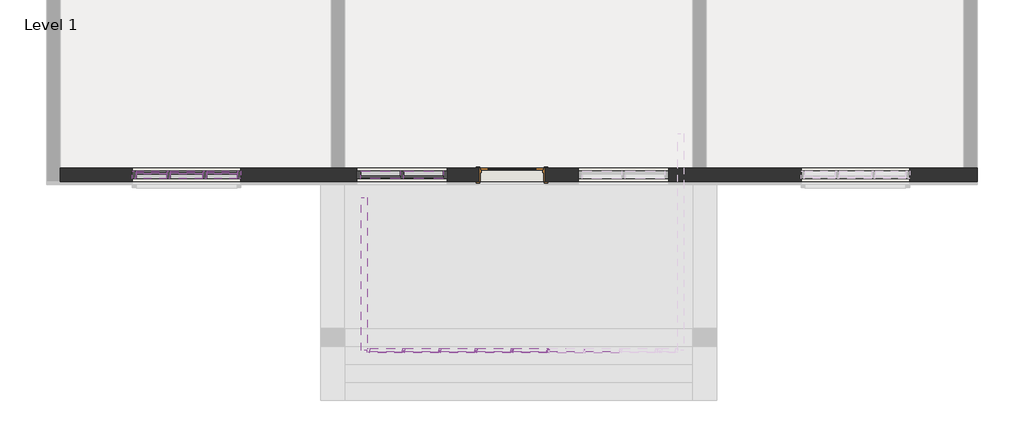
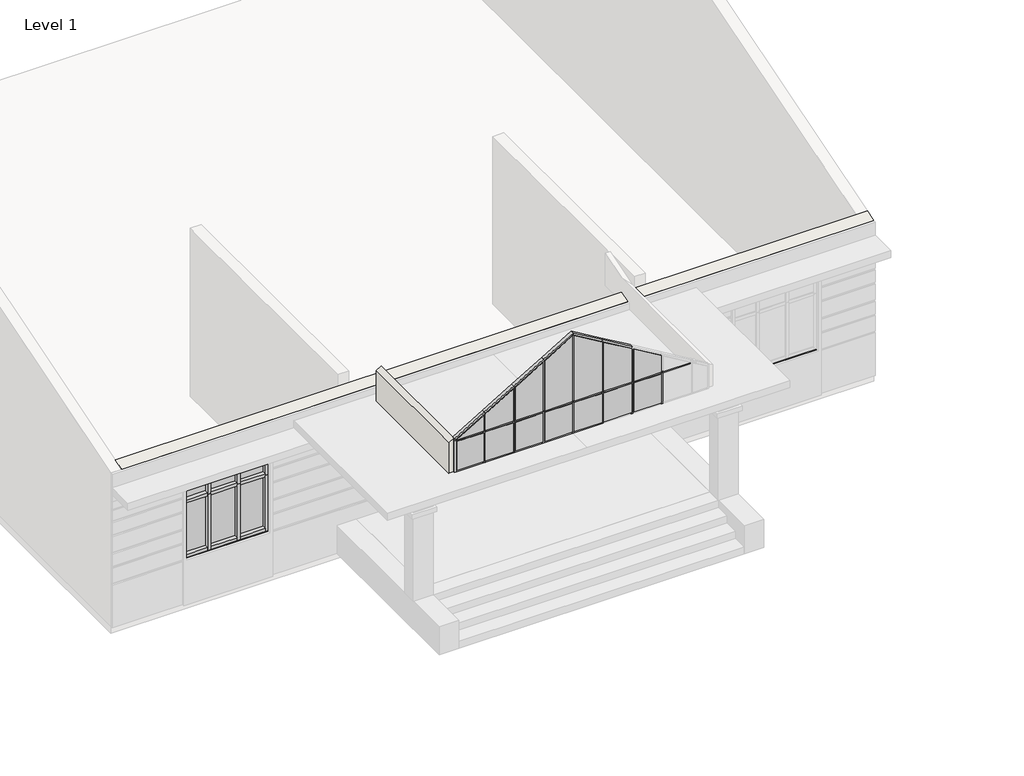
# One storey, part 1 of 2: 57 members, 22 plates, 2 walls, 1 door.
"""IFC4 building model written with IfcOpenShell, lengths in millimetres."""

from ifc_helpers import new_model, si_unit, frame, origin, place, context, project, spatial, polyline, outline, extrude, faceted_brep, transform, mapped, element, save
from components import door_103cf79b, member_83e1ecc3, member_06c20982, member_b8e7570c, member_bb410062, member_6458fcce, member_a67f877f, member_c8158400, member_1ba99afd, member_594eddbe, member_3c184fc8, member_ff75f20c, member_eb314aa0, member_ee25ef0f, member_c8c782b1, member_99569e28, member_7b64f847, member_0b7646a3, member_2b49869a, member_aaa03826, member_0a1a1ade, member_a980948f, member_6e77e263, member_47bfaf8a, member_75074519, member_c33c434a, member_38e9bff8, member_062c1ce8, system_panel_glazed_d796fc41, system_panel_glazed_2d0a2ff2, system_panel_glazed_c086748d, system_panel_glazed_4278ab3a, system_panel_glazed_31f7001e, system_panel_glazed_f02c31ce, system_panel_glazed_0f57d06b, system_panel_glazed_ee2a426c, system_panel_glazed_65593f79, system_panel_glazed_0e80e67f, system_panel_glazed_cec062fa, system_panel_glazed_9c640d8a, system_panel_glazed_3d703fd1, system_panel_glazed_02eac8f9

model = new_model("IFC4")

# Units and contexts
model_context = context("Model", 3, world=origin())
ifc_project = project(units=[si_unit("LENGTHUNIT", "METRE", prefix="MILLI")], contexts=[model_context])

# Site, building, storey
site = spatial("IfcSite", under=ifc_project)
building = spatial("IfcBuilding", under=site)
storey = spatial("IfcBuildingStorey", under=building, Name="Level 1", Elevation=0.0)

# Door
placement = place(None, origin())
door_shape = door_103cf79b(model_context)
element("IfcDoor", 1, ObjectType="Door-Interior-Single-1_Panel-Wood : 3'6\" x 7'", at=placement, inside=storey, context=model_context, shape_type="MappedRepresentation", body=[
    mapped(door_shape, transform((-905.7652342, -1559.6844336, 584.2), x_axis=(1.0, 0.0, 0.0), y_axis=(0.0, 1.0, 0.0), z_axis=(0.0, 0.0, 1.0))),
])

# Members
member_shape = member_83e1ecc3(model_context)
element("IfcMember", 2, ObjectType="Rectangular Mullion : 1.5\" x 2.5\" rectangular", at=placement, inside=storey, context=model_context, shape_type="MappedRepresentation", body=[
    mapped(member_shape, transform((-905.7652342, -4522.7940778, 5385.8290246), x_axis=(0.5109163571310298, 0.0, 0.8596304299034313), y_axis=(0.0, 1.0, 0.0), z_axis=(-0.8596304299034313, 0.0, 0.5109163571310298))),
])
member_2_shape = member_06c20982(model_context)
element("IfcMember", 3, ObjectType="Rectangular Mullion : 1.5\" x 2.5\" rectangular", at=placement, inside=storey, context=model_context, shape_type="MappedRepresentation", body=[
    mapped(member_2_shape, transform((-3345.0817556, -4522.7940778, 3936.0354067), x_axis=(-0.5109163571310278, 0.0, 0.8596304299034325), y_axis=(0.0, 1.0, 0.0), z_axis=(-0.8596304299034324, 0.0, -0.5109163571310277))),
])
member_3_shape = member_b8e7570c(model_context)
element("IfcMember", 4, ObjectType="Rectangular Mullion : 1.5\" x 2.5\" rectangular", at=placement, inside=storey, context=model_context, shape_type="MappedRepresentation", body=[
    mapped(member_3_shape, transform((-1496.3152342, -4522.7940778, 3886.2), x_axis=(0.0, 0.0, 1.0), y_axis=(0.0, 1.0, 0.0), z_axis=(-1.0, 0.0, 0.0))),
])
element("IfcMember", 5, ObjectType="Rectangular Mullion : 1.5\" x 2.5\" rectangular", at=placement, inside=storey, context=model_context, shape_type="MappedRepresentation", body=[
    mapped(member_3_shape, transform((-886.7152342, -4522.7940778, 3886.2), x_axis=(0.0, 0.0, 1.0), y_axis=(0.0, 1.0, 0.0), z_axis=(-1.0, 0.0, 0.0))),
])
element("IfcMember", 6, ObjectType="Rectangular Mullion : 1.5\" x 2.5\" rectangular", at=placement, inside=storey, context=model_context, shape_type="MappedRepresentation", body=[
    mapped(member_3_shape, transform((-277.1152342, -4522.7940778, 3886.2), x_axis=(0.0, 0.0, 1.0), y_axis=(0.0, 1.0, 0.0), z_axis=(-1.0, 0.0, 0.0))),
])
element("IfcMember", 7, ObjectType="Rectangular Mullion : 1.5\" x 2.5\" rectangular", at=placement, inside=storey, context=model_context, shape_type="MappedRepresentation", body=[
    mapped(member_3_shape, transform((332.4847658, -4522.7940778, 3886.2), x_axis=(0.0, 0.0, 1.0), y_axis=(0.0, 1.0, 0.0), z_axis=(-1.0, 0.0, 0.0))),
])
element("IfcMember", 8, ObjectType="Rectangular Mullion : 1.5\" x 2.5\" rectangular", at=placement, inside=storey, context=model_context, shape_type="MappedRepresentation", body=[
    mapped(member_3_shape, transform((942.0847658, -4522.7940778, 3886.2), x_axis=(0.0, 0.0, 1.0), y_axis=(0.0, 1.0, 0.0), z_axis=(-1.0, 0.0, 0.0))),
])
element("IfcMember", 9, ObjectType="Rectangular Mullion : 1.5\" x 2.5\" rectangular", at=placement, inside=storey, context=model_context, shape_type="MappedRepresentation", body=[
    mapped(member_3_shape, transform((-2105.9152342, -4522.7940778, 3886.2), x_axis=(0.0, 0.0, 1.0), y_axis=(0.0, 1.0, 0.0), z_axis=(-1.0, 0.0, 0.0))),
])
element("IfcMember", 10, ObjectType="Rectangular Mullion : 1.5\" x 2.5\" rectangular", at=placement, inside=storey, context=model_context, shape_type="MappedRepresentation", body=[
    mapped(member_3_shape, transform((-2715.5152342, -4522.7940778, 3886.2), x_axis=(0.0, 0.0, 1.0), y_axis=(0.0, 1.0, 0.0), z_axis=(-1.0, 0.0, 0.0))),
])
member_4_shape = member_bb410062(model_context)
element("IfcMember", 11, ObjectType="Rectangular Mullion : 1.5\" x 2.5\" rectangular", at=placement, inside=storey, context=model_context, shape_type="MappedRepresentation", body=[
    mapped(member_4_shape, transform((-3306.9817556, -4522.7940778, 3886.2), x_axis=(0.0, 0.0, 1.0), y_axis=(0.0, 1.0, 0.0), z_axis=(-1.0, 0.0, 0.0))),
])
member_5_shape = member_6458fcce(model_context)
element("IfcMember", 12, ObjectType="Rectangular Mullion : 1.5\" x 2.5\" rectangular", at=placement, inside=storey, context=model_context, shape_type="MappedRepresentation", body=[
    mapped(member_5_shape, transform((-905.7652342, -4522.7940778, 3200.4), x_axis=(-1.0, 0.0, 0.0), y_axis=(0.0, 1.0, 0.0), z_axis=(0.0, 0.0, -1.0))),
])
element("IfcMember", 13, ObjectType="Rectangular Mullion : 1.5\" x 2.5\" rectangular", at=placement, inside=storey, context=model_context, shape_type="MappedRepresentation", body=[
    mapped(member_5_shape, transform((-296.1652342, -4522.7940778, 3200.4), x_axis=(-1.0, 0.0, 0.0), y_axis=(0.0, 1.0, 0.0), z_axis=(0.0, 0.0, -1.0))),
])
element("IfcMember", 14, ObjectType="Rectangular Mullion : 1.5\" x 2.5\" rectangular", at=placement, inside=storey, context=model_context, shape_type="MappedRepresentation", body=[
    mapped(member_5_shape, transform((313.4347658, -4522.7940778, 3200.4), x_axis=(-1.0, 0.0, 0.0), y_axis=(0.0, 1.0, 0.0), z_axis=(0.0, 0.0, -1.0))),
])
element("IfcMember", 15, ObjectType="Rectangular Mullion : 1.5\" x 2.5\" rectangular", at=placement, inside=storey, context=model_context, shape_type="MappedRepresentation", body=[
    mapped(member_5_shape, transform((923.0347658, -4522.7940778, 3200.4), x_axis=(-1.0, 0.0, 0.0), y_axis=(0.0, 1.0, 0.0), z_axis=(0.0, 0.0, -1.0))),
])
element("IfcMember", 16, ObjectType="Rectangular Mullion : 1.5\" x 2.5\" rectangular", at=placement, inside=storey, context=model_context, shape_type="MappedRepresentation", body=[
    mapped(member_5_shape, transform((-1515.3652342, -4522.7940778, 3200.4), x_axis=(-1.0, 0.0, 0.0), y_axis=(0.0, 1.0, 0.0), z_axis=(0.0, 0.0, -1.0))),
])
element("IfcMember", 17, ObjectType="Rectangular Mullion : 1.5\" x 2.5\" rectangular", at=placement, inside=storey, context=model_context, shape_type="MappedRepresentation", body=[
    mapped(member_5_shape, transform((-2124.9652342, -4522.7940778, 3200.4), x_axis=(-1.0, 0.0, 0.0), y_axis=(0.0, 1.0, 0.0), z_axis=(0.0, 0.0, -1.0))),
])
element("IfcMember", 18, ObjectType="Rectangular Mullion : 1.5\" x 2.5\" rectangular", at=placement, inside=storey, context=model_context, shape_type="MappedRepresentation", body=[
    mapped(member_5_shape, transform((-2734.5652342, -4522.7940778, 3200.4), x_axis=(-1.0, 0.0, 0.0), y_axis=(0.0, 1.0, 0.0), z_axis=(0.0, 0.0, -1.0))),
])
member_6_shape = member_a67f877f(model_context)
element("IfcMember", 19, ObjectType="Rectangular Mullion : 1.5\" x 2.5\" rectangular", at=placement, inside=storey, context=model_context, shape_type="MappedRepresentation", body=[
    mapped(member_6_shape, transform((-924.8152342, -4522.7940778, 3200.4), x_axis=(0.0, 0.0, -1.0), y_axis=(0.0, 1.0, 0.0), z_axis=(1.0, 0.0, 0.0))),
])
element("IfcMember", 20, ObjectType="Rectangular Mullion : 1.5\" x 2.5\" rectangular", at=placement, inside=storey, context=model_context, shape_type="MappedRepresentation", body=[
    mapped(member_6_shape, transform((-315.2152342, -4522.7940778, 3200.4), x_axis=(0.0, 0.0, -1.0), y_axis=(0.0, 1.0, 0.0), z_axis=(1.0, 0.0, 0.0))),
])
element("IfcMember", 21, ObjectType="Rectangular Mullion : 1.5\" x 2.5\" rectangular", at=placement, inside=storey, context=model_context, shape_type="MappedRepresentation", body=[
    mapped(member_6_shape, transform((-1534.4152342, -4522.7940778, 3200.4), x_axis=(0.0, 0.0, -1.0), y_axis=(0.0, 1.0, 0.0), z_axis=(1.0, 0.0, 0.0))),
])
element("IfcMember", 22, ObjectType="Rectangular Mullion : 1.5\" x 2.5\" rectangular", at=placement, inside=storey, context=model_context, shape_type="MappedRepresentation", body=[
    mapped(member_6_shape, transform((-2144.0152342, -4522.7940778, 3200.4), x_axis=(0.0, 0.0, -1.0), y_axis=(0.0, 1.0, 0.0), z_axis=(1.0, 0.0, 0.0))),
])
member_7_shape = member_c8158400(model_context)
element("IfcMember", 23, ObjectType="Rectangular Mullion : 1.5\" x 2.5\" rectangular", at=placement, inside=storey, context=model_context, shape_type="MappedRepresentation", body=[
    mapped(member_7_shape, transform((-2753.6152342, -4522.7940778, 3200.4), x_axis=(0.0, 0.0, -1.0), y_axis=(0.0, 1.0, 0.0), z_axis=(1.0, 0.0, 0.0))),
])
member_8_shape = member_1ba99afd(model_context)
element("IfcMember", 24, ObjectType="Rectangular Mullion : 1.5\" x 2.5\" rectangular", at=placement, inside=storey, context=model_context, shape_type="MappedRepresentation", body=[
    mapped(member_8_shape, transform((-1515.3652342, -4522.7940778, 5023.5168024), x_axis=(-0.5109163571310282, 0.0, 0.8596304299034321), y_axis=(0.0, 1.0, 0.0), z_axis=(-0.8596304299034323, 0.0, -0.5109163571310283))),
])
member_9_shape = member_594eddbe(model_context)
element("IfcMember", 25, ObjectType="Rectangular Mullion : 1.5\" x 2.5\" rectangular", at=placement, inside=storey, context=model_context, shape_type="MappedRepresentation", body=[
    mapped(member_9_shape, transform((-2124.9652342, -4522.7940778, 4661.2045803), x_axis=(-0.5109163571310272, 0.0, 0.8596304299034329), y_axis=(0.0, 1.0, 0.0), z_axis=(-0.8596304299034327, 0.0, -0.5109163571310271))),
])
element("IfcMember", 26, ObjectType="Rectangular Mullion : 1.5\" x 2.5\" rectangular", at=placement, inside=storey, context=model_context, shape_type="MappedRepresentation", body=[
    mapped(member_9_shape, transform((-2734.5652342, -4522.7940778, 4298.8923581), x_axis=(-0.5109163571310278, 0.0, 0.8596304299034325), y_axis=(0.0, 1.0, 0.0), z_axis=(-0.8596304299034325, 0.0, -0.5109163571310278))),
])
element("IfcMember", 27, ObjectType="Rectangular Mullion : 1.5\" x 2.5\" rectangular", at=placement, inside=storey, context=model_context, shape_type="MappedRepresentation", body=[
    mapped(member_9_shape, transform((-296.1652342, -4522.7940778, 5023.5168024), x_axis=(0.5109163571310306, 0.0, 0.8596304299034309), y_axis=(0.0, 1.0, 0.0), z_axis=(-0.8596304299034307, 0.0, 0.5109163571310305))),
])
member_10_shape = member_3c184fc8(model_context)
element("IfcMember", 28, ObjectType="Rectangular Mullion : 1.5\" x 2.5\" rectangular", at=placement, inside=storey, context=model_context, shape_type="MappedRepresentation", body=[
    mapped(member_10_shape, transform((-905.7652342, -4522.7940778, 3886.2), x_axis=(-1.0, 0.0, 0.0), y_axis=(0.0, 1.0, 0.0), z_axis=(0.0, 0.0, -1.0))),
])
member_11_shape = member_ff75f20c(model_context)
element("IfcMember", 29, ObjectType="Rectangular Mullion : 1.5\" x 2.5\" rectangular", at=placement, inside=storey, context=model_context, shape_type="MappedRepresentation", body=[
    mapped(member_11_shape, transform((-296.1652342, -4522.7940778, 3886.2), x_axis=(-1.0, 0.0, 0.0), y_axis=(0.0, 1.0, 0.0), z_axis=(0.0, 0.0, -1.0))),
])
member_12_shape = member_eb314aa0(model_context)
element("IfcMember", 30, ObjectType="Rectangular Mullion : 1.5\" x 2.5\" rectangular", at=placement, inside=storey, context=model_context, shape_type="MappedRepresentation", body=[
    mapped(member_12_shape, transform((-1515.3652342, -4522.7940778, 3886.2), x_axis=(-1.0, 0.0, 0.0), y_axis=(0.0, 1.0, 0.0), z_axis=(0.0, 0.0, -1.0))),
])
member_13_shape = member_ee25ef0f(model_context)
element("IfcMember", 31, ObjectType="Rectangular Mullion : 1.5\" x 2.5\" rectangular", at=placement, inside=storey, context=model_context, shape_type="MappedRepresentation", body=[
    mapped(member_13_shape, transform((-2124.9652342, -4522.7940778, 3886.2), x_axis=(-1.0, 0.0, 0.0), y_axis=(0.0, 1.0, 0.0), z_axis=(0.0, 0.0, -1.0))),
])
member_14_shape = member_c8c782b1(model_context)
element("IfcMember", 32, ObjectType="Rectangular Mullion : 1.5\" x 2.5\" rectangular", at=placement, inside=storey, context=model_context, shape_type="MappedRepresentation", body=[
    mapped(member_14_shape, transform((-2734.5652342, -4522.7940778, 3886.2), x_axis=(-1.0, 0.0, 0.0), y_axis=(0.0, 1.0, 0.0), z_axis=(0.0, 0.0, -1.0))),
])
member_15_shape = member_99569e28(model_context)
element("IfcMember", 33, ObjectType="Rectangular Mullion : 1.5\" x 2.5\" rectangular", at=placement, inside=storey, context=model_context, shape_type="MappedRepresentation", body=[
    mapped(member_15_shape, transform((-3345.0817556, -4522.7940778, 3200.4), x_axis=(-1.0, 0.0, 0.0), y_axis=(0.0, 1.0, 0.0), z_axis=(0.0, 0.0, -1.0))),
])
member_16_shape = member_7b64f847(model_context)
element("IfcMember", 34, ObjectType="Rectangular Mullion : 1.5\" x 2.5\" rectangular", at=placement, inside=storey, context=model_context, shape_type="MappedRepresentation", body=[
    mapped(member_16_shape, transform((-3345.0817556, -4522.7940778, 3886.2), x_axis=(-1.0, 0.0, 0.0), y_axis=(0.0, 1.0, 0.0), z_axis=(0.0, 0.0, -1.0))),
])
member_17_shape = member_0b7646a3(model_context)
element("IfcMember", 35, ObjectType="Rectangular Mullion : 2.5\" x 5\" rectangular", at=placement, inside=storey, context=model_context, shape_type="MappedRepresentation", body=[
    mapped(member_17_shape, transform((-5541.2652342, -1562.8594336, 2743.2), x_axis=(0.0, 0.0, 1.0), y_axis=(0.0, -1.0, 0.0), z_axis=(1.0, 0.0, 0.0))),
])
element("IfcMember", 36, ObjectType="Rectangular Mullion : 2.5\" x 5\" rectangular", at=placement, inside=storey, context=model_context, shape_type="MappedRepresentation", body=[
    mapped(member_17_shape, transform((-6728.7152342, -1562.8594336, 2743.2), x_axis=(0.0, 0.0, 1.0), y_axis=(0.0, -1.0, 0.0), z_axis=(1.0, 0.0, 0.0))),
])
element("IfcMember", 37, ObjectType="Rectangular Mullion : 2.5\" x 5\" rectangular", at=placement, inside=storey, context=model_context, shape_type="MappedRepresentation", body=[
    mapped(member_17_shape, transform((-7243.0652342, -1562.8594336, 914.4), x_axis=(0.0, 0.0, -1.0), y_axis=(0.0, -1.0, 0.0), z_axis=(-1.0, 0.0, 0.0))),
])
element("IfcMember", 38, ObjectType="Rectangular Mullion : 2.5\" x 5\" rectangular", at=placement, inside=storey, context=model_context, shape_type="MappedRepresentation", body=[
    mapped(member_17_shape, transform((-6055.6152342, -1562.8594336, 914.4), x_axis=(0.0, 0.0, -1.0), y_axis=(0.0, -1.0, 0.0), z_axis=(-1.0, 0.0, 0.0))),
])
member_18_shape = member_2b49869a(model_context)
element("IfcMember", 39, ObjectType="Rectangular Mullion : 2.5\" x 5\" rectangular", at=placement, inside=storey, context=model_context, shape_type="MappedRepresentation", body=[
    mapped(member_18_shape, transform((-6696.9652342, -1562.8594336, 914.4), x_axis=(1.0, 0.0, 0.0), y_axis=(0.0, -1.0, 0.0), z_axis=(0.0, 0.0, -1.0))),
])
element("IfcMember", 40, ObjectType="Rectangular Mullion : 2.5\" x 5\" rectangular", at=placement, inside=storey, context=model_context, shape_type="MappedRepresentation", body=[
    mapped(member_18_shape, transform((-6087.3652342, -1562.8594336, 914.4), x_axis=(1.0, 0.0, 0.0), y_axis=(0.0, -1.0, 0.0), z_axis=(0.0, 0.0, -1.0))),
])
member_19_shape = member_aaa03826(model_context)
element("IfcMember", 41, ObjectType="Rectangular Mullion : 2.5\" x 5\" rectangular", at=placement, inside=storey, context=model_context, shape_type="MappedRepresentation", body=[
    mapped(member_19_shape, transform((-6728.7152342, -1562.8594336, 2133.6), x_axis=(0.0, 0.0, 1.0), y_axis=(0.0, -1.0, 0.0), z_axis=(1.0, 0.0, 0.0))),
])
element("IfcMember", 42, ObjectType="Rectangular Mullion : 2.5\" x 5\" rectangular", at=placement, inside=storey, context=model_context, shape_type="MappedRepresentation", body=[
    mapped(member_19_shape, transform((-5541.2652342, -1562.8594336, 2133.6), x_axis=(0.0, 0.0, 1.0), y_axis=(0.0, -1.0, 0.0), z_axis=(1.0, 0.0, 0.0))),
])
member_20_shape = member_0a1a1ade(model_context)
element("IfcMember", 43, ObjectType="Rectangular Mullion : 2.5\" x 5\" rectangular", at=placement, inside=storey, context=model_context, shape_type="MappedRepresentation", body=[
    mapped(member_20_shape, transform((-6119.1152342, -1562.8594336, 2133.6), x_axis=(0.0, 0.0, 1.0), y_axis=(0.0, -1.0, 0.0), z_axis=(1.0, 0.0, 0.0))),
])
member_21_shape = member_a980948f(model_context)
element("IfcMember", 44, ObjectType="Rectangular Mullion : 2.5\" x 5\" rectangular", at=placement, inside=storey, context=model_context, shape_type="MappedRepresentation", body=[
    mapped(member_21_shape, transform((-6665.2152342, -1562.8594336, 914.4), x_axis=(0.0, 0.0, -1.0), y_axis=(0.0, -1.0, 0.0), z_axis=(-1.0, 0.0, 0.0))),
])
element("IfcMember", 45, ObjectType="Rectangular Mullion : 2.5\" x 5\" rectangular", at=placement, inside=storey, context=model_context, shape_type="MappedRepresentation", body=[
    mapped(member_21_shape, transform((-6119.1152342, -1562.8594336, 2743.2), x_axis=(0.0, 0.0, 1.0), y_axis=(0.0, -1.0, 0.0), z_axis=(1.0, 0.0, 0.0))),
])
member_22_shape = member_6e77e263(model_context)
element("IfcMember", 46, ObjectType="Rectangular Mullion : 2.5\" x 5\" rectangular", at=placement, inside=storey, context=model_context, shape_type="MappedRepresentation", body=[
    mapped(member_22_shape, transform((-6696.9652342, -1562.8594336, 2133.6), x_axis=(1.0, 0.0, 0.0), y_axis=(0.0, -1.0, 0.0), z_axis=(0.0, 0.0, -1.0))),
])
element("IfcMember", 47, ObjectType="Rectangular Mullion : 2.5\" x 5\" rectangular", at=placement, inside=storey, context=model_context, shape_type="MappedRepresentation", body=[
    mapped(member_22_shape, transform((-6087.3652342, -1562.8594336, 2133.6), x_axis=(1.0, 0.0, 0.0), y_axis=(0.0, -1.0, 0.0), z_axis=(0.0, 0.0, -1.0))),
])
member_23_shape = member_47bfaf8a(model_context)
element("IfcMember", 48, ObjectType="Rectangular Mullion : 2.5\" x 5\" rectangular", at=placement, inside=storey, context=model_context, shape_type="MappedRepresentation", body=[
    mapped(member_23_shape, transform((-7306.5652342, -1562.8594336, 2743.2), x_axis=(-1.0, 0.0, 0.0), y_axis=(0.0, -1.0, 0.0), z_axis=(0.0, 0.0, 1.0))),
])
member_24_shape = member_75074519(model_context)
element("IfcMember", 49, ObjectType="Rectangular Mullion : 2.5\" x 5\" rectangular", at=placement, inside=storey, context=model_context, shape_type="MappedRepresentation", body=[
    mapped(member_24_shape, transform((-5477.7652342, -1562.8594336, 914.4), x_axis=(1.0, 0.0, 0.0), y_axis=(0.0, -1.0, 0.0), z_axis=(0.0, 0.0, -1.0))),
])
element("IfcMember", 50, ObjectType="Rectangular Mullion : 2.5\" x 5\" rectangular", at=placement, inside=storey, context=model_context, shape_type="MappedRepresentation", body=[
    mapped(member_23_shape, transform((-5477.7652342, -1562.8594336, 2133.6), x_axis=(1.0, 0.0, 0.0), y_axis=(0.0, -1.0, 0.0), z_axis=(0.0, 0.0, -1.0))),
])
element("IfcMember", 51, ObjectType="Rectangular Mullion : 2.5\" x 5\" rectangular", at=placement, inside=storey, context=model_context, shape_type="MappedRepresentation", body=[
    mapped(member_24_shape, transform((-7306.5652342, -1562.8594336, 2133.6), x_axis=(-1.0, 0.0, 0.0), y_axis=(0.0, -1.0, 0.0), z_axis=(0.0, 0.0, 1.0))),
])
member_25_shape = member_c33c434a(model_context)
element("IfcMember", 52, ObjectType="Rectangular Mullion : 2.5\" x 5\" rectangular", at=placement, inside=storey, context=model_context, shape_type="MappedRepresentation", body=[
    mapped(member_25_shape, transform((-3458.4652342, -1562.8594336, 2743.2), x_axis=(0.0, 0.0, 1.0), y_axis=(0.0, 1.0, 0.0), z_axis=(-1.0, 0.0, 0.0))),
])
element("IfcMember", 53, ObjectType="Rectangular Mullion : 2.5\" x 5\" rectangular", at=placement, inside=storey, context=model_context, shape_type="MappedRepresentation", body=[
    mapped(member_25_shape, transform((-2728.2152342, -1562.8594336, 2743.2), x_axis=(0.0, 0.0, 1.0), y_axis=(0.0, 1.0, 0.0), z_axis=(-1.0, 0.0, 0.0))),
])
element("IfcMember", 54, ObjectType="Rectangular Mullion : 2.5\" x 5\" rectangular", at=placement, inside=storey, context=model_context, shape_type="MappedRepresentation", body=[
    mapped(member_25_shape, transform((-2061.4652342, -1562.8594336, 1066.8), x_axis=(0.0, 0.0, -1.0), y_axis=(0.0, 1.0, 0.0), z_axis=(1.0, 0.0, 0.0))),
])
element("IfcMember", 55, ObjectType="Rectangular Mullion : 2.5\" x 5\" rectangular", at=placement, inside=storey, context=model_context, shape_type="MappedRepresentation", body=[
    mapped(member_25_shape, transform((-2791.7152342, -1562.8594336, 1066.8), x_axis=(0.0, 0.0, -1.0), y_axis=(0.0, 1.0, 0.0), z_axis=(1.0, 0.0, 0.0))),
])
member_26_shape = member_38e9bff8(model_context)
element("IfcMember", 56, ObjectType="Rectangular Mullion : 2.5\" x 5\" rectangular", at=placement, inside=storey, context=model_context, shape_type="MappedRepresentation", body=[
    mapped(member_26_shape, transform((-2759.9652342, -1562.8594336, 1066.8), x_axis=(-1.0, 0.0, 0.0), y_axis=(0.0, 1.0, 0.0), z_axis=(0.0, 0.0, -1.0))),
])
member_27_shape = member_062c1ce8(model_context)
element("IfcMember", 57, ObjectType="Rectangular Mullion : 2.5\" x 5\" rectangular", at=placement, inside=storey, context=model_context, shape_type="MappedRepresentation", body=[
    mapped(member_27_shape, transform((-1997.9652342, -1562.8594336, 2743.2), x_axis=(1.0, 0.0, 0.0), y_axis=(0.0, 1.0, 0.0), z_axis=(0.0, 0.0, 1.0))),
])
element("IfcMember", 58, ObjectType="Rectangular Mullion : 2.5\" x 5\" rectangular", at=placement, inside=storey, context=model_context, shape_type="MappedRepresentation", body=[
    mapped(member_27_shape, transform((-3521.9652342, -1562.8594336, 1066.8), x_axis=(-1.0, 0.0, 0.0), y_axis=(0.0, 1.0, 0.0), z_axis=(0.0, 0.0, -1.0))),
])

# Plates
system_panel_glazed_shape = system_panel_glazed_d796fc41(model_context)
element("IfcPlate", 59, ObjectType="System Panel : Glazed", at=placement, inside=storey, context=model_context, shape_type="MappedRepresentation", body=[
    mapped(system_panel_glazed_shape, transform((-6985.8902342, -1562.8594336, 977.9), x_axis=(1.0, 0.0, 0.0), y_axis=(0.0, 1.0, 0.0), z_axis=(0.0, 0.0, 1.0))),
])
element("IfcPlate", 60, ObjectType="System Panel : Glazed", at=placement, inside=storey, context=model_context, shape_type="MappedRepresentation", body=[
    mapped(system_panel_glazed_shape, transform((-5798.4402342, -1562.8594336, 977.9), x_axis=(1.0, 0.0, 0.0), y_axis=(0.0, 1.0, 0.0), z_axis=(0.0, 0.0, 1.0))),
])
system_panel_glazed_2_shape = system_panel_glazed_2d0a2ff2(model_context)
element("IfcPlate", 61, ObjectType="System Panel : Glazed", at=placement, inside=storey, context=model_context, shape_type="MappedRepresentation", body=[
    mapped(system_panel_glazed_2_shape, transform((-6392.1652342, -1562.8594336, 977.9), x_axis=(1.0, 0.0, 0.0), y_axis=(0.0, 1.0, 0.0), z_axis=(0.0, 0.0, 1.0))),
])
system_panel_glazed_3_shape = system_panel_glazed_c086748d(model_context)
element("IfcPlate", 62, ObjectType="System Panel : Glazed", at=placement, inside=storey, context=model_context, shape_type="MappedRepresentation", body=[
    mapped(system_panel_glazed_3_shape, transform((-6985.8902342, -1562.8594336, 2165.35), x_axis=(1.0, 0.0, 0.0), y_axis=(0.0, 1.0, 0.0), z_axis=(0.0, 0.0, 1.0))),
])
element("IfcPlate", 63, ObjectType="System Panel : Glazed", at=placement, inside=storey, context=model_context, shape_type="MappedRepresentation", body=[
    mapped(system_panel_glazed_3_shape, transform((-5798.4402342, -1562.8594336, 2165.35), x_axis=(1.0, 0.0, 0.0), y_axis=(0.0, 1.0, 0.0), z_axis=(0.0, 0.0, 1.0))),
])
system_panel_glazed_4_shape = system_panel_glazed_4278ab3a(model_context)
element("IfcPlate", 64, ObjectType="System Panel : Glazed", at=placement, inside=storey, context=model_context, shape_type="MappedRepresentation", body=[
    mapped(system_panel_glazed_4_shape, transform((-6392.1652342, -1562.8594336, 2165.35), x_axis=(1.0, 0.0, 0.0), y_axis=(0.0, 1.0, 0.0), z_axis=(0.0, 0.0, 1.0))),
])
system_panel_glazed_5_shape = system_panel_glazed_31f7001e(model_context)
element("IfcPlate", 65, ObjectType="System Panel : Glazed", at=placement, inside=storey, context=model_context, shape_type="MappedRepresentation", body=[
    mapped(system_panel_glazed_5_shape, transform((-2394.8402342, -1562.8594336, 1130.3), x_axis=(-1.0, 0.0, 0.0), y_axis=(0.0, -1.0, 0.0), z_axis=(0.0, 0.0, 1.0))),
])
element("IfcPlate", 66, ObjectType="System Panel : Glazed", at=placement, inside=storey, context=model_context, shape_type="MappedRepresentation", body=[
    mapped(system_panel_glazed_5_shape, transform((-3125.0902342, -1562.8594336, 1130.3), x_axis=(-1.0, 0.0, 0.0), y_axis=(0.0, -1.0, 0.0), z_axis=(0.0, 0.0, 1.0))),
])
system_panel_glazed_6_shape = system_panel_glazed_f02c31ce(model_context)
element("IfcPlate", 67, ObjectType="System Panel : Glazed", at=placement, inside=storey, context=model_context, shape_type="MappedRepresentation", body=[
    mapped(system_panel_glazed_6_shape, transform((-1210.5652342, -4522.7940778, 3238.5), x_axis=(-1.0, 0.0, 0.0), y_axis=(0.0, -1.0, 0.0), z_axis=(0.0, 0.0, 1.0))),
])
element("IfcPlate", 68, ObjectType="System Panel : Glazed", at=placement, inside=storey, context=model_context, shape_type="MappedRepresentation", body=[
    mapped(system_panel_glazed_6_shape, transform((-600.9652342, -4522.7940778, 3238.5), x_axis=(-1.0, 0.0, 0.0), y_axis=(0.0, -1.0, 0.0), z_axis=(0.0, 0.0, 1.0))),
])
element("IfcPlate", 69, ObjectType="System Panel : Glazed", at=placement, inside=storey, context=model_context, shape_type="MappedRepresentation", body=[
    mapped(system_panel_glazed_6_shape, transform((8.6347658, -4522.7940778, 3238.5), x_axis=(-1.0, 0.0, 0.0), y_axis=(0.0, -1.0, 0.0), z_axis=(0.0, 0.0, 1.0))),
])
element("IfcPlate", 70, ObjectType="System Panel : Glazed", at=placement, inside=storey, context=model_context, shape_type="MappedRepresentation", body=[
    mapped(system_panel_glazed_6_shape, transform((618.2347658, -4522.7940778, 3238.5), x_axis=(-1.0, 0.0, 0.0), y_axis=(0.0, -1.0, 0.0), z_axis=(0.0, 0.0, 1.0))),
])
element("IfcPlate", 71, ObjectType="System Panel : Glazed", at=placement, inside=storey, context=model_context, shape_type="MappedRepresentation", body=[
    mapped(system_panel_glazed_6_shape, transform((-1820.1652342, -4522.7940778, 3238.5), x_axis=(-1.0, 0.0, 0.0), y_axis=(0.0, -1.0, 0.0), z_axis=(0.0, 0.0, 1.0))),
])
element("IfcPlate", 72, ObjectType="System Panel : Glazed", at=placement, inside=storey, context=model_context, shape_type="MappedRepresentation", body=[
    mapped(system_panel_glazed_6_shape, transform((-2429.7652342, -4522.7940778, 3238.5), x_axis=(-1.0, 0.0, 0.0), y_axis=(0.0, -1.0, 0.0), z_axis=(0.0, 0.0, 1.0))),
])
system_panel_glazed_7_shape = system_panel_glazed_0f57d06b(model_context)
element("IfcPlate", 73, ObjectType="System Panel : Glazed", at=placement, inside=storey, context=model_context, shape_type="MappedRepresentation", body=[
    mapped(system_panel_glazed_7_shape, transform((-1210.5652342, -4522.7940778, 3905.25), x_axis=(-1.0, 0.0, 0.0), y_axis=(0.0, -1.0, 0.0), z_axis=(0.0, 0.0, 1.0))),
])
system_panel_glazed_8_shape = system_panel_glazed_ee2a426c(model_context)
element("IfcPlate", 74, ObjectType="System Panel : Glazed", at=placement, inside=storey, context=model_context, shape_type="MappedRepresentation", body=[
    mapped(system_panel_glazed_8_shape, transform((-600.9652342, -4522.7940778, 3905.25), x_axis=(-1.0, 0.0, 0.0), y_axis=(0.0, -1.0, 0.0), z_axis=(0.0, 0.0, 1.0))),
])
system_panel_glazed_9_shape = system_panel_glazed_65593f79(model_context)
element("IfcPlate", 75, ObjectType="System Panel : Glazed", at=placement, inside=storey, context=model_context, shape_type="MappedRepresentation", body=[
    mapped(system_panel_glazed_9_shape, transform((8.6347658, -4522.7940778, 3905.25), x_axis=(-1.0, 0.0, 0.0), y_axis=(0.0, -1.0, 0.0), z_axis=(0.0, 0.0, 1.0))),
])
system_panel_glazed_10_shape = system_panel_glazed_0e80e67f(model_context)
element("IfcPlate", 76, ObjectType="System Panel : Glazed", at=placement, inside=storey, context=model_context, shape_type="MappedRepresentation", body=[
    mapped(system_panel_glazed_10_shape, transform((618.2347658, -4522.7940778, 3905.25), x_axis=(-1.0, 0.0, 0.0), y_axis=(0.0, -1.0, 0.0), z_axis=(0.0, 0.0, 1.0))),
])
system_panel_glazed_11_shape = system_panel_glazed_cec062fa(model_context)
element("IfcPlate", 77, ObjectType="System Panel : Glazed", at=placement, inside=storey, context=model_context, shape_type="MappedRepresentation", body=[
    mapped(system_panel_glazed_11_shape, transform((-1820.1652342, -4522.7940778, 3905.25), x_axis=(-1.0, 0.0, 0.0), y_axis=(0.0, -1.0, 0.0), z_axis=(0.0, 0.0, 1.0))),
])
system_panel_glazed_12_shape = system_panel_glazed_9c640d8a(model_context)
element("IfcPlate", 78, ObjectType="System Panel : Glazed", at=placement, inside=storey, context=model_context, shape_type="MappedRepresentation", body=[
    mapped(system_panel_glazed_12_shape, transform((-2429.7652342, -4522.7940778, 3905.25), x_axis=(-1.0, 0.0, 0.0), y_axis=(0.0, -1.0, 0.0), z_axis=(0.0, 0.0, 1.0))),
])
system_panel_glazed_13_shape = system_panel_glazed_3d703fd1(model_context)
element("IfcPlate", 79, ObjectType="System Panel : Glazed", at=placement, inside=storey, context=model_context, shape_type="MappedRepresentation", body=[
    mapped(system_panel_glazed_13_shape, transform((-3030.2984949, -4522.7940778, 3238.5), x_axis=(-1.0, 0.0, 0.0), y_axis=(0.0, -1.0, 0.0), z_axis=(0.0, 0.0, 1.0))),
])
system_panel_glazed_14_shape = system_panel_glazed_02eac8f9(model_context)
element("IfcPlate", 80, ObjectType="System Panel : Glazed", at=placement, inside=storey, context=model_context, shape_type="MappedRepresentation", body=[
    mapped(system_panel_glazed_14_shape, transform((-3030.2984949, -4522.7940778, 3905.25), x_axis=(-1.0, 0.0, 0.0), y_axis=(0.0, -1.0, 0.0), z_axis=(0.0, 0.0, 1.0))),
])

# Walls
element("IfcWall", 81, ObjectType="4\" wall", at=placement, inside=storey, context=model_context, shape_type="SweptSolid", body=[
    extrude(outline(polyline([(3200.4, -3345.0817556), (3936.0354067, -3345.0817556), (3875.6500363, -3446.6817556), (3200.4, -3446.6817556), (3200.4, -3345.0817556)])), frame((0.0, -4522.7940778, 0.0), z_axis=(0.0, 1.0, 0.0), x_axis=(0.0, 0.0, 1.0)), (0.0, 0.0, 1.0), 2581.3276166),
])
element("IfcWall", 82, ObjectType="9\"", at=placement, inside=storey, context=model_context, shape_type="Brep", body=[
    faceted_brep([(6942.8347658, -1448.5594336, 0.0), (6714.2347658, -1448.5594336, 0.0), (2370.8347658, -1448.5594336, 0.0), (2142.2347658, -1448.5594336, 0.0), (-3725.1652342, -1448.5594336, 0.0), (-3953.7652342, -1448.5594336, 0.0), (-8525.7652342, -1448.5594336, 0.0), (-8525.7652342, -1448.5594336, 3408.7631864), (1887.3182444, -1448.5594336, 3408.7631864), (1988.9182444, -1448.5594336, 3408.7631864), (6714.2347658, -1448.5594336, 3408.7631864), (6942.8347658, -1448.5594336, 3408.7631864), (-346.9652342, -1448.5594336, 584.2), (-346.9652342, -1448.5594336, 2743.2), (-1464.5652342, -1448.5594336, 2743.2), (-1464.5652342, -1448.5594336, 584.2), (-1997.9652342, -1448.5594336, 1066.8), (-1997.9652342, -1448.5594336, 2743.2), (-3521.9652342, -1448.5594336, 2743.2), (-3521.9652342, -1448.5594336, 1066.8), (211.8347658, -1448.5594336, 2743.2), (211.8347658, -1448.5594336, 1066.8), (1735.8347658, -1448.5594336, 1066.8), (1735.8347658, -1448.5594336, 2743.2), (-7306.5652342, -1448.5594336, 2743.2), (-7306.5652342, -1448.5594336, 914.4), (-5477.7652342, -1448.5594336, 914.4), (-5477.7652342, -1448.5594336, 2743.2), (5799.8347658, -1448.5594336, 914.4), (5799.8347658, -1448.5594336, 2743.2), (3971.0347658, -1448.5594336, 2743.2), (3971.0347658, -1448.5594336, 914.4), (-8525.7652342, -1677.1594336, 0.0), (6942.8347658, -1677.1594336, 0.0), (6942.8347658, -1677.1594336, 3338.8731526), (1988.9182444, -1677.1594336, 3338.8731526), (1887.3182444, -1677.1594336, 3338.8731526), (-8525.7652342, -1677.1594336, 3338.8731526), (-346.9652342, -1677.1594336, 2743.2), (-346.9652342, -1677.1594336, 584.2), (-1464.5652342, -1677.1594336, 584.2), (-1464.5652342, -1677.1594336, 2743.2), (-1997.9652342, -1677.1594336, 2743.2), (-1997.9652342, -1677.1594336, 1066.8), (-3521.9652342, -1677.1594336, 1066.8), (-3521.9652342, -1677.1594336, 2743.2), (211.8347658, -1677.1594336, 1066.8), (211.8347658, -1677.1594336, 2743.2), (1735.8347658, -1677.1594336, 2743.2), (1735.8347658, -1677.1594336, 1066.8), (-7306.5652342, -1677.1594336, 914.4), (-7306.5652342, -1677.1594336, 2743.2), (-5477.7652342, -1677.1594336, 2743.2), (-5477.7652342, -1677.1594336, 914.4), (5799.8347658, -1677.1594336, 2743.2), (5799.8347658, -1677.1594336, 914.4), (3971.0347658, -1677.1594336, 914.4), (3971.0347658, -1677.1594336, 2743.2)], [[[0, 1, 2, 3, 4, 5, 6, 7, 8, 9, 10, 11], [12, 13, 14, 15], [16, 17, 18, 19], [20, 21, 22, 23], [24, 25, 26, 27], [28, 29, 30, 31]], [[32, 33, 34, 35, 36, 37], [38, 39, 40, 41], [42, 43, 44, 45], [46, 47, 48, 49], [50, 51, 52, 53], [54, 55, 56, 57]], [[6, 5, 4, 3, 2, 1, 0, 33, 32]], [[0, 11, 34, 33]], [[7, 6, 32, 37]], [[12, 39, 38, 13]], [[13, 38, 41, 14]], [[40, 15, 14, 41]], [[39, 12, 15, 40]], [[42, 17, 16, 43]], [[17, 42, 45, 18]], [[18, 45, 44, 19]], [[43, 16, 19, 44]], [[46, 21, 20, 47]], [[47, 20, 23, 48]], [[48, 23, 22, 49]], [[21, 46, 49, 22]], [[50, 25, 24, 51]], [[51, 24, 27, 52]], [[52, 27, 26, 53]], [[25, 50, 53, 26]], [[28, 55, 54, 29]], [[29, 54, 57, 30]], [[30, 57, 56, 31]], [[55, 28, 31, 56]], [[11, 10, 9, 8, 7, 37, 36, 35, 34]]]),
])

save(model, "model.ifc")

# Revit data of these elements
# Type "Door-Interior-Single-1_Panel-Wood : 3'6\" x 7'"
#   Type Mark = "9"
#   Assembly Code = "C1020300"
#   Analytic Construction = "Wooden"
#   Top Rail = 0' - 4 11/16"
#   Thickness = 0' - 1 3/8"
#   Thermal Resistance (R) = 2.5876 (h·ft²·°F)/BTU
#   Swing Angle [instance default] = 90.00°
#   Stiles = 0' - 4 3/4"
#   Rough Width = 3' - 8"
#   Rough Height = 7' - 1"
#   Height = 7' - 0"
#   Width = 3' - 6"
#   Heat Transfer Coefficient (U) = 0.3865 BTU/(h·ft²·°F)
#   Bottom Rail = 0' - 9 1/8"
#   Trim Material = Cherry
#   Panel Material = Cherry
#   Frame Material = Cherry
#   Door Handle Material = Aluminum
#   Visual Light Transmittance = 0
#   Solar Heat Gain Coefficient = 0
#   Wall Closure = (empty or 0)
#   Function = (empty or 0)
# Type "Rectangular Mullion : 1.5\" x 2.5\" rectangular"
#   built-in parameter 1007304 = 0.208333 (stored number, unit not read)
#   built-in parameter 1007301 = 0.0625 (stored number, unit not read)
#   built-in parameter 1007300 = 0.0625 (stored number, unit not read)
# Type "Rectangular Mullion : 2.5\" x 5\" rectangular"
#   built-in parameter 1007304 = 0.416667 (stored number, unit not read)
#   built-in parameter 1007301 = 0.104167 (stored number, unit not read)
#   built-in parameter 1007300 = 0.104167 (stored number, unit not read)
# Type "System Panel : Glazed"
#   Construction Type Id = "GSP4R"
#   Analytic Construction = "1/8 in Pilkington single glazing"
#   Visual Light Transmittance = 0.9
#   Solar Heat Gain Coefficient = 0.86
#   Heat Transfer Coefficient (U) = 1.18115 BTU/(h·ft²·°F)
#   Define Thermal Properties by = 1
# Type "4\" wall"
#   Assembly Code = "B2010"
#   Layers, outside or top first: 0' - 4" "Gypsum Wall Board" (function 1)
# Type "9\""
#   Assembly Code = "B2010"
#   Layers, outside or top first: 0' - 9" "Gypsum Wall Board" (function 1)
# Element 1 (IfcDoor, "Door-Interior-Single-1_Panel-Wood : 3'6\" x 7'")
#   Swing Angle = 90.00°
#   Phase Created = New Construction
#   Materials on its faces: "Cherry", "Aluminum"
# Elements 2, 3, 4, 5, 6, 7, 8, 9, 10, 11, 12, 13, 14, 15, 16, 17, 18, 19, 20, 21, 22, 23, 24, 25, 26, 27, 28, 29, 30, 31, 32, 33, 34 (IfcMember, "Rectangular Mullion : 1.5\" x 2.5\" rectangular")
#   Phase Created = New Construction
# Elements 35, 36, 37, 38, 39, 40, 41, 42, 43, 44, 45, 46, 47, 48, 49, 50, 51, 52, 53, 54, 55, 56, 57, 58 (IfcMember, "Rectangular Mullion : 2.5\" x 5\" rectangular")
#   Phase Created = New Construction
# Elements 59, 60, 61, 62, 63, 64, 65, 66, 67, 68, 69, 70, 71, 72, 73, 74, 75, 76, 77, 78, 79, 80 (IfcPlate, "System Panel : Glazed")
#   Phase Created = New Construction
#   Materials on its faces: "Glass"
# Element 81 (IfcWall, "4\" wall")
#   built-in parameter 1001111 = 10' - 6"
#   Top Offset = -3' - 0"
#   Base Offset = 10' - 6"
#   wall height = 7' - 0"
#   Phase Created = New Construction
#   Base Constraint = Level 1
#   Top Constraint = Level 2
#   Materials on its faces: "Gypsum Wall Board"
# Element 82 (IfcWall, "9\"")
#   Top Offset = 0' - 0"
#   Base Offset = 0' - 0"
#   wall height = 12' - 0"
#   Phase Created = New Construction
#   Base Constraint = Level 1
#   Top Constraint = Level 2
#   Materials on its faces: "Gypsum Wall Board"
# Materials
#   "Cherry": class "Wood", colour RGB 226 177 128, transparency 0, Description = "Prunus Serotina", Cost = 0
#   "Aluminum": class "Metal", colour RGB 247 247 247, transparency 0, Description = "Aluminum 6061", Cost = 0
#   "Gypsum Wall Board": class "Generic", colour RGB 127 127 127, transparency 0, Description = "Gypsum Wall Board", Cost = 0
#   "Glass": class "Glass", colour RGB 0 128 192, transparency 0.75, Description = "Soda Lime Glass", Cost = 0
